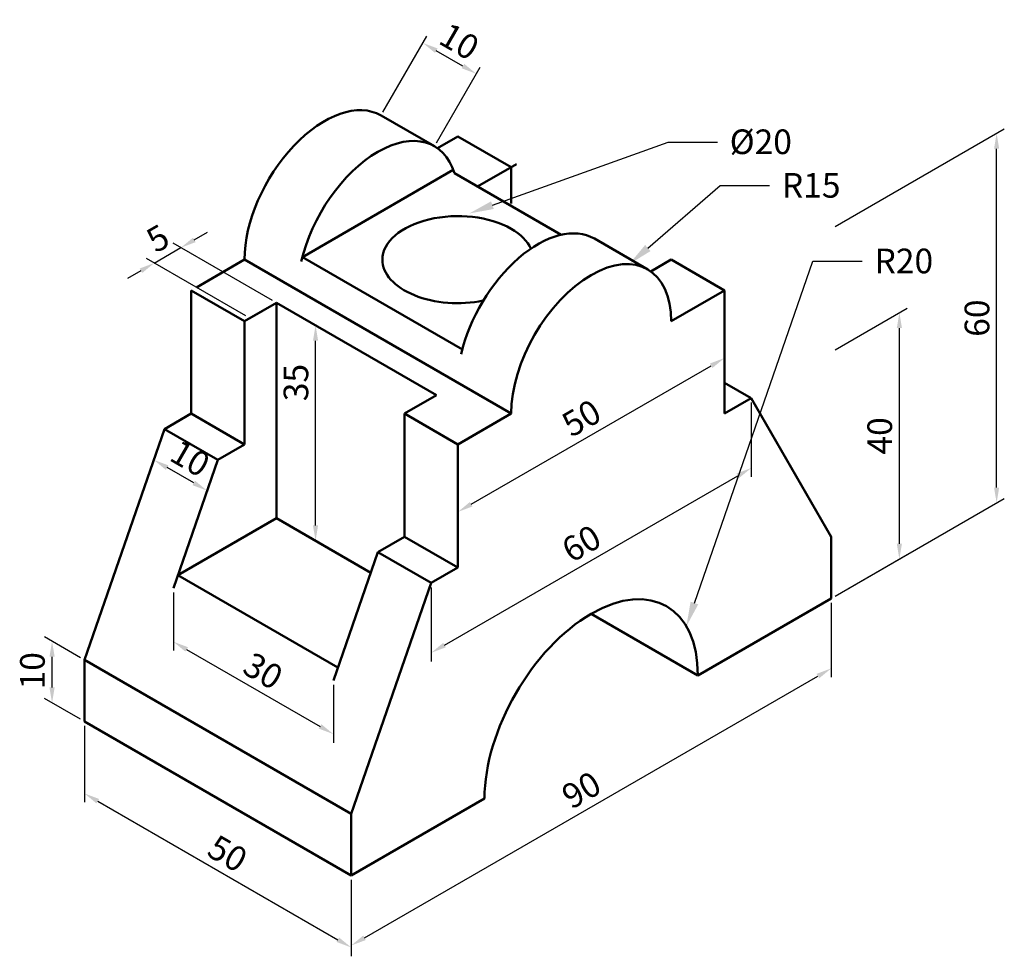
# Model space of a CAD drawing. Units: millimetres. Extents: x 1718 to 1878, y 1929 to 2081.
import ezdxf
from ezdxf import colors
from ezdxf.entities.mleader import LeaderData, LeaderLine
from ezdxf.math import Vec2, Vec3

# ---------------------------------------------------------------- set-up
doc = ezdxf.new("R2010")
doc.units = ezdxf.units.MM
for name, color, linetype, lineweight in [('M-DIMS', 2, 'Continuous', 25), ('M-OUTL', 7, 'Continuous', 50), ('M-TEXT', 3, 'Continuous', 25)]:
    doc.layers.add(name, color=color, linetype=linetype, lineweight=lineweight)
doc.styles.get("Standard").update_dxf_attribs({"font": 'arial.ttf'})
doc.dimstyles.new('ISO-25', dxfattribs={"dimtxt": 4, "dimasz": 2.5, "dimexe": 1.25, "dimexo": 0.625, "dimtad": 1, "dimtxsty": 'Standard', "dimcen": 2.5, "dimadec": 0, "dimazin": 0, "dimtfac": 1, "dimtmove": 0, "dimatfit": 3, "dimfxl": 1, "dimarcsym": 0})

# ---------------------------------------------------------------- blocks, each defined once
blk = doc.blocks.new('*D1')
at = {"layer": 'Defpoints', "color": 0, "transparency": 16777216}
for p in [(1729.01, 1966.68), (1772.31, 1941.68), (1772.31, 1930)]:
    blk.add_point(p, dxfattribs=at)
at = {"layer": 'M-DIMS', "color": 0, "lineweight": -2, "transparency": 16777216}
for p, q in [((1729.01, 1965.96), (1729.01, 1953.56)), ((1731.17, 1953.75), (1770.14, 1931.25)), ((1772.31, 1940.96), (1772.31, 1928.56))]:
    blk.add_line(p, q, dxfattribs=at)
at = {"layer": 'M-DIMS', "color": 0, "transparency": 16777216}
for points in [[(1731.38, 1954.11), (1730.96, 1953.39), (1729.01, 1955)], [(1770.35, 1931.61), (1769.93, 1930.89), (1772.31, 1930)]]:
    blk.add_solid(points, dxfattribs=at)
at = {"layer": 'M-DIMS', "color": 0, "transparency": 16777216, "insert": (1751.99, 1944.81), "char_height": 4, "attachment_point": 5, "rotation": 330}
blk.add_mtext('50', dxfattribs=at)
blk = doc.blocks.new('*D2')
at = {"layer": 'Defpoints', "color": 0, "transparency": 16777216}
for p in [(1850.25, 1986.68), (1850.25, 1975.31), (1772.31, 1941.68)]:
    blk.add_point(p, dxfattribs=at)
at = {"layer": 'M-DIMS', "color": 0, "lineweight": -2, "transparency": 16777216}
for p, q in [((1850.25, 1985.96), (1850.25, 1973.87)), ((1774.47, 1931.56), (1848.08, 1974.06)), ((1772.31, 1940.96), (1772.31, 1928.87))]:
    blk.add_line(p, q, dxfattribs=at)
at = {"layer": 'M-DIMS', "color": 0, "transparency": 16777216}
for points in [[(1847.88, 1974.42), (1848.29, 1973.7), (1850.25, 1975.31)], [(1774.26, 1931.92), (1774.68, 1931.2), (1772.31, 1930.31)]]:
    blk.add_solid(points, dxfattribs=at)
at = {"layer": 'M-DIMS', "color": 0, "transparency": 16777216, "insert": (1809.94, 1955.12), "char_height": 4, "attachment_point": 5, "rotation": 30}
blk.add_mtext('90', dxfattribs=at)
blk = doc.blocks.new('*D3')
at = {"layer": 'Defpoints', "color": 0, "transparency": 16777216}
for p in [(1723.75, 1979.71), (1729.01, 1976.68), (1729.01, 1966.68)]:
    blk.add_point(p, dxfattribs=at)
at = {"layer": 'M-DIMS', "color": 0, "lineweight": -2, "transparency": 16777216}
for p, q in [((1728.38, 1977.04), (1722.5, 1980.43)), ((1723.75, 1972.21), (1723.75, 1977.21)), ((1728.38, 1967.04), (1722.5, 1970.43))]:
    blk.add_line(p, q, dxfattribs=at)
at = {"layer": 'M-DIMS', "color": 0, "transparency": 16777216}
for points in [[(1723.33, 1977.21), (1724.17, 1977.21), (1723.75, 1979.71)], [(1723.33, 1972.21), (1724.17, 1972.21), (1723.75, 1969.71)]]:
    blk.add_solid(points, dxfattribs=at)
at = {"layer": 'M-DIMS', "color": 0, "transparency": 16777216, "insert": (1721.08, 1974.92), "char_height": 4, "attachment_point": 5, "rotation": 90}
blk.add_mtext('10', dxfattribs=at)
blk = doc.blocks.new('*D4')
at = {"layer": 'Defpoints', "color": 0, "transparency": 16777216}
for p in [(1877.1, 2062.18), (1850.25, 2046.68), (1850.25, 1986.68)]:
    blk.add_point(p, dxfattribs=at)
at = {"layer": 'M-DIMS', "color": 0, "lineweight": -2, "transparency": 16777216}
for p, q in [((1850.87, 2047.04), (1878.35, 2062.9)), ((1877.1, 2004.68), (1877.1, 2059.68)), ((1850.87, 1987.04), (1878.35, 2002.9))]:
    blk.add_line(p, q, dxfattribs=at)
at = {"layer": 'M-DIMS', "color": 0, "transparency": 16777216}
for points in [[(1876.68, 2059.68), (1877.51, 2059.68), (1877.1, 2062.18)], [(1876.68, 2004.68), (1877.51, 2004.68), (1877.1, 2002.18)]]:
    blk.add_solid(points, dxfattribs=at)
at = {"layer": 'M-DIMS', "color": 0, "transparency": 16777216, "insert": (1874.43, 2032.18), "char_height": 4, "attachment_point": 5, "rotation": 90}
blk.add_mtext('60', dxfattribs=at)
blk = doc.blocks.new('*D5')
at = {"layer": 'Defpoints', "color": 0, "transparency": 16777216}
for p in [(1861.31, 2033.06), (1850.25, 2026.68), (1850.25, 1986.68)]:
    blk.add_point(p, dxfattribs=at)
at = {"layer": 'M-DIMS', "color": 0, "lineweight": -2, "transparency": 16777216}
for p, q in [((1850.87, 2027.04), (1862.56, 2033.79)), ((1861.31, 1995.56), (1861.31, 2030.56)), ((1850.87, 1987.04), (1862.56, 1993.79))]:
    blk.add_line(p, q, dxfattribs=at)
at = {"layer": 'M-DIMS', "color": 0, "transparency": 16777216}
for points in [[(1860.89, 2030.56), (1861.73, 2030.56), (1861.31, 2033.06)], [(1860.89, 1995.56), (1861.73, 1995.56), (1861.31, 1993.06)]]:
    blk.add_solid(points, dxfattribs=at)
at = {"layer": 'M-DIMS', "color": 0, "transparency": 16777216, "insert": (1858.64, 2013.06), "char_height": 4, "attachment_point": 5, "rotation": 90}
blk.add_mtext('40', dxfattribs=at)
blk = doc.blocks.new('*D6')
at = {"layer": 'Defpoints', "color": 0, "transparency": 16777216}
for p in [(1837.26, 2019.18), (1837.26, 2007.84), (1785.3, 1989.18)]:
    blk.add_point(p, dxfattribs=at)
at = {"layer": 'M-DIMS', "color": 0, "lineweight": -2, "transparency": 16777216}
for p, q in [((1837.26, 2018.46), (1837.26, 2006.4)), ((1787.46, 1979.09), (1835.09, 2006.59)), ((1785.3, 1988.46), (1785.3, 1976.4))]:
    blk.add_line(p, q, dxfattribs=at)
at = {"layer": 'M-DIMS', "color": 0, "transparency": 16777216}
for points in [[(1834.89, 2006.95), (1835.3, 2006.23), (1837.26, 2007.84)], [(1787.25, 1979.45), (1787.67, 1978.73), (1785.3, 1977.84)]]:
    blk.add_solid(points, dxfattribs=at)
at = {"layer": 'M-DIMS', "color": 0, "transparency": 16777216, "insert": (1809.94, 1995.15), "char_height": 4, "attachment_point": 5, "rotation": 30}
blk.add_mtext('60', dxfattribs=at)
blk = doc.blocks.new('*D7')
at = {"layer": 'Defpoints', "color": 0, "transparency": 16777216}
for p in [(1832.93, 2036.68), (1832.93, 2025.71), (1789.63, 2011.68)]:
    blk.add_point(p, dxfattribs=at)
at = {"layer": 'M-DIMS', "color": 0, "lineweight": -2, "transparency": 16777216}
for p, q in [((1832.93, 2035.96), (1832.93, 2024.27)), ((1791.79, 2001.96), (1830.76, 2024.46)), ((1789.63, 2010.96), (1789.63, 1999.27))]:
    blk.add_line(p, q, dxfattribs=at)
at = {"layer": 'M-DIMS', "color": 0, "transparency": 16777216}
for points in [[(1830.56, 2024.82), (1830.97, 2024.1), (1832.93, 2025.71)], [(1791.58, 2002.32), (1792, 2001.6), (1789.63, 2000.71)]]:
    blk.add_solid(points, dxfattribs=at)
at = {"layer": 'M-DIMS', "color": 0, "transparency": 16777216, "insert": (1809.94, 2015.52), "char_height": 4, "attachment_point": 5, "rotation": 30}
blk.add_mtext('50', dxfattribs=at)
blk = doc.blocks.new('*D8')
at = {"layer": 'Defpoints', "color": 0, "transparency": 16777216}
for p in [(1744.67, 2043.63), (1760.18, 2034.68), (1755.85, 2032.18)]:
    blk.add_point(p, dxfattribs=at)
at = {"layer": 'M-DIMS', "color": 0, "lineweight": -2, "transparency": 16777216}
for p, q in [((1746.84, 2044.88), (1749, 2046.13)), ((1740.34, 2041.13), (1744.67, 2043.63)), ((1759.56, 2035.04), (1743.42, 2044.35)), ((1755.23, 2032.54), (1739.09, 2041.85)), ((1738.18, 2039.88), (1736.01, 2038.63))]:
    blk.add_line(p, q, dxfattribs=at)
at = {"layer": 'M-DIMS', "color": 0, "transparency": 16777216}
for points in [[(1746.63, 2045.24), (1747.05, 2044.52), (1744.67, 2043.63)], [(1737.97, 2040.24), (1738.39, 2039.52), (1740.34, 2041.13)]]:
    blk.add_solid(points, dxfattribs=at)
at = {"layer": 'M-DIMS', "color": 0, "transparency": 16777216, "insert": (1741.18, 2044.69), "char_height": 4, "attachment_point": 5, "rotation": 30}
blk.add_mtext('5', dxfattribs=at)
blk = doc.blocks.new('*D9')
at = {"layer": 'Defpoints', "color": 0, "transparency": 16777216}
for p in [(1743.44, 1988.35), (1769.42, 1973.35), (1769.42, 1964.64)]:
    blk.add_point(p, dxfattribs=at)
at = {"layer": 'M-DIMS', "color": 0, "lineweight": -2, "transparency": 16777216}
for p, q in [((1743.44, 1987.62), (1743.44, 1978.2)), ((1745.6, 1978.39), (1767.26, 1965.89)), ((1769.42, 1972.62), (1769.42, 1963.2))]:
    blk.add_line(p, q, dxfattribs=at)
at = {"layer": 'M-DIMS', "color": 0, "transparency": 16777216}
for points in [[(1745.81, 1978.75), (1745.4, 1978.03), (1743.44, 1979.64)], [(1767.46, 1966.25), (1767.05, 1965.53), (1769.42, 1964.64)]]:
    blk.add_solid(points, dxfattribs=at)
at = {"layer": 'M-DIMS', "color": 0, "transparency": 16777216, "insert": (1757.76, 1974.45), "char_height": 4, "attachment_point": 5, "rotation": 330}
blk.add_mtext('30', dxfattribs=at)
blk = doc.blocks.new('*D10')
at = {"layer": 'Defpoints', "color": 0, "transparency": 16777216}
for p in [(1783.96, 2076.86), (1777.16, 2065.09), (1785.82, 2060.09)]:
    blk.add_point(p, dxfattribs=at)
at = {"layer": 'M-DIMS', "color": 0, "lineweight": -2, "transparency": 16777216}
for p, q in [((1777.47, 2065.63), (1784.58, 2077.94)), ((1790.45, 2073.11), (1786.12, 2075.61)), ((1786.14, 2060.63), (1793.24, 2072.94))]:
    blk.add_line(p, q, dxfattribs=at)
at = {"layer": 'M-DIMS', "color": 0, "transparency": 16777216}
for points in [[(1786.33, 2075.97), (1785.92, 2075.25), (1783.96, 2076.86)], [(1790.66, 2073.47), (1790.25, 2072.75), (1792.62, 2071.86)]]:
    blk.add_solid(points, dxfattribs=at)
at = {"layer": 'M-DIMS', "color": 0, "transparency": 16777216, "insert": (1789.62, 2076.67), "char_height": 4, "attachment_point": 5, "rotation": 330}
blk.add_mtext('10', dxfattribs=at)
blk = doc.blocks.new('*D11')
at = {"layer": 'Defpoints', "color": 0, "transparency": 16777216}
for p in [(1760.18, 2034.68), (1766.53, 2031.02), (1760.18, 1999.68)]:
    blk.add_point(p, dxfattribs=at)
at = {"layer": 'M-DIMS', "color": 0, "lineweight": -2, "transparency": 16777216}
for p, q in [((1760.81, 2034.32), (1767.78, 2030.3)), ((1766.53, 1998.52), (1766.53, 2028.52)), ((1760.81, 1999.32), (1767.78, 1995.3))]:
    blk.add_line(p, q, dxfattribs=at)
at = {"layer": 'M-DIMS', "color": 0, "transparency": 16777216}
for points in [[(1766.11, 2028.52), (1766.94, 2028.52), (1766.53, 2031.02)], [(1766.11, 1998.52), (1766.94, 1998.52), (1766.53, 1996.02)]]:
    blk.add_solid(points, dxfattribs=at)
at = {"layer": 'M-DIMS', "color": 0, "transparency": 16777216, "insert": (1763.86, 2021.72), "char_height": 4, "attachment_point": 5, "rotation": 90}
blk.add_mtext('35', dxfattribs=at)
blk = doc.blocks.new('*D12')
at = {"layer": 'Defpoints', "color": 0, "transparency": 16777216}
for p in [(1742, 2014.18), (1740.26, 2009.17), (1750.66, 2009.18)]:
    blk.add_point(p, dxfattribs=at)
at = {"layer": 'M-DIMS', "color": 0, "lineweight": -2, "transparency": 16777216}
for p, q in [((1741.79, 2013.58), (1739.84, 2007.96)), ((1746.75, 2005.42), (1742.42, 2007.92)), ((1750.45, 2008.58), (1748.5, 2002.96))]:
    blk.add_line(p, q, dxfattribs=at)
at = {"layer": 'M-DIMS', "color": 0, "transparency": 16777216}
for points in [[(1742.63, 2008.28), (1742.22, 2007.55), (1740.26, 2009.17)], [(1746.96, 2005.78), (1746.55, 2005.05), (1748.92, 2004.17)]]:
    blk.add_solid(points, dxfattribs=at)
at = {"layer": 'M-DIMS', "color": 0, "transparency": 16777216, "insert": (1745.92, 2008.98), "char_height": 4, "attachment_point": 5, "rotation": 330}
blk.add_mtext('10', dxfattribs=at)

msp = doc.modelspace()

# ---------------------------------------------------------------- linework, layer by layer
at = {"layer": 'M-OUTL'}
for p, q in [((1777.162, 2065.089), (1785.823, 2060.089)), ((1789.628, 2061.679), (1786.32, 2059.769)), ((1798.288, 2056.679), (1789.628, 2061.679)), ((1764.39, 2042.108), (1788.885, 2056.25)), ((1789.068, 2055.71), (1806.389, 2045.71)), ((1799.154, 2057.179), (1792.839, 2053.533)), ((1798.288, 2050.821), (1798.288, 2056.679)), ((1811.803, 2045.089), (1820.464, 2040.089)), ((1747.192, 2037.179), (1754.986, 2041.679)), ((1747.192, 2037.179), (1754.986, 2041.679)), ((1754.986, 2041.679), (1798.288, 2016.679)), ((1764.39, 2042.108), (1790.371, 2027.108)), ((1824.268, 2041.679), (1820.96, 2039.769)), ((1832.929, 2036.679), (1824.268, 2041.679)), ((1754.987, 2031.679), (1746.326, 2036.679)), ((1746.326, 2036.679), (1746.326, 2016.679)), ((1832.929, 2036.679), (1824.268, 2031.679)), ((1832.929, 2036.679), (1832.929, 2016.679)), ((1760.183, 2034.679), (1754.987, 2031.679)), ((1760.183, 2034.679), (1755.852, 2032.179)), ((1786.163, 2019.679), (1760.183, 2034.679)), ((1760.183, 2034.679), (1760.183, 1999.679)), ((1754.987, 2031.679), (1754.987, 2011.679)), ((1837.259, 2019.179), (1832.929, 2021.679)), ((1780.967, 2016.679), (1786.163, 2019.679)), ((1832.929, 2016.679), (1837.259, 2019.179)), ((1837.259, 2019.179), (1850.249, 1996.679)), ((1741.996, 2014.179), (1746.326, 2016.679)), ((1746.326, 2016.679), (1754.986, 2011.679)), ((1789.627, 2011.679), (1780.967, 2016.679)), ((1780.967, 2016.679), (1780.967, 1996.679)), ((1798.288, 2016.679), (1789.627, 2011.679)), ((1741.996, 2014.179), (1729.006, 1976.679)), ((1750.656, 2009.179), (1741.996, 2014.179)), ((1754.986, 2011.679), (1750.656, 2009.179)), ((1789.627, 2011.679), (1789.627, 1991.679)), ((1750.656, 2009.179), (1743.439, 1988.346)), ((1744.161, 1990.429), (1760.183, 1999.679)), ((1775.482, 1990.846), (1760.183, 1999.679)), ((1776.637, 1994.179), (1780.967, 1996.679)), ((1780.967, 1996.679), (1789.627, 1991.679)), ((1850.249, 1986.679), (1850.249, 1996.679)), ((1776.637, 1994.179), (1769.42, 1973.346)), ((1785.297, 1989.179), (1776.637, 1994.179)), ((1770.142, 1975.429), (1744.161, 1990.429)), ((1789.627, 1991.679), (1785.297, 1989.179)), ((1785.297, 1989.179), (1772.307, 1951.679)), ((1828.599, 1974.179), (1850.249, 1986.679)), ((1828.599, 1974.179), (1811.278, 1984.179)), ((1772.307, 1951.679), (1729.006, 1976.679)), ((1729.006, 1976.679), (1729.006, 1966.679)), ((1729.006, 1966.679), (1772.307, 1941.679)), ((1772.307, 1941.679), (1793.958, 1954.179)), ((1772.307, 1941.679), (1772.307, 1951.679))]:
    msp.add_line(p, q, dxfattribs=at)
for centre, major_axis, start_param, end_param in [((1767.977, 2049.179), (-9.186, -15.91), 3.1415927, 5.4977871), ((1776.637, 2044.179), (-9.186, -15.91), 2.65071, 5.2032717), ((1789.628, 2041.679), (12.247, 0), 0.7853982, 3.1415927), ((1802.618, 2029.179), (-9.186, -15.91), 3.1415927, 5.2032717), ((1789.628, 2041.679), (12.247, 0), 0.255112, 0.7853982), ((1811.278, 2024.179), (-9.186, -15.91), 2.3561945, 5.4977871), ((1789.628, 2041.679), (12.247, 0), 3.1415927, 5.0557077), ((1811.278, 1964.179), (-12.247, -21.213), 2.3561945, 5.4977871)]:
    msp.add_ellipse(centre, major_axis=major_axis, ratio=0.5773503, start_param=start_param, end_param=end_param, dxfattribs=at)

# ---------------------------------------------------------------- dimensions: what is measured, and where the dimension line sits
at = {"layer": 'M-DIMS'}
for p1, p2, distance, picture, middle in [((1785.823, 2060.089), (1777.162, 2065.089), -13.593, '*D10', (1789.623, 2076.671)), ((1850.249, 1986.679), (1850.249, 2046.679), -26.847, '*D4', (1874.429, 2032.179)), ((1755.852, 2032.179), (1760.183, 2034.679), 15.508, '*D8', (1741.18, 2044.686)), ((1789.627, 2011.679), (1832.929, 2036.679), -9.497, '*D7', (1809.944, 2015.523)), ((1850.249, 1986.679), (1850.249, 2026.679), -11.059, '*D5', (1858.641, 2013.064)), ((1785.297, 1989.179), (1837.259, 2019.179), -9.819, '*D6', (1809.944, 1995.151)), ((1750.656, 2009.179), (1741.996, 2014.179), 5.21, '*D12', (1745.923, 2008.975)), ((1743.439, 1988.346), (1769.42, 1973.346), -7.539, '*D9', (1757.764, 1974.452)), ((1772.307, 1941.679), (1850.249, 1986.679), -9.843, '*D2', (1809.944, 1955.124)), ((1729.006, 1966.679), (1772.307, 1941.679), -10.115, '*D1', (1751.99, 1944.809))]:
    dim = msp.add_aligned_dim(p1=p1, p2=p2, distance=distance, dimstyle='ISO-25', override={"dimclrd": 0, "dimclre": 0, "dimclrt": 0}, dxfattribs=at)
    dim.commit()
    dim.dimension.update_dxf_attribs({"geometry": picture, "text_midpoint": middle})
for base, p1, p2, picture, middle in [((1766.526, 2031.017), (1760.183, 1999.679), (1760.183, 2034.679), '*D11', (1766.526, 2021.724)), ((1723.751, 1979.713), (1729.006, 1966.679), (1729.006, 1976.679), '*D3', (1723.751, 1974.919))]:
    dim = msp.add_linear_dim(base=base, p1=p1, p2=p2, angle=90, dimstyle='ISO-25', override={"dimclrd": 0, "dimclre": 0, "dimclrt": 0}, dxfattribs=at)
    dim.commit()
    dim.dimension.update_dxf_attribs({"geometry": picture, "text_midpoint": middle, "dimtype": 161})

# ---------------------------------------------------------------- leaders
at = {"layer": 'M-TEXT'}
ml = msp.add_multileader_mtext('Standard', dxfattribs=at)
ml.set_content('%%C20', color=256)
ml.set_leader_properties()
ml.build(insert=Vec2(0, 0))
ctx = ml.context
ctx.base_point, ctx.plane_origin = Vec3(1831.759, 2060.739), Vec3(1791.481, 2042.103)
notes = []
notes.append((ctx, [(0, (1, 1, 0), (1823.759, 2060.739), (1, 0), 8, [(0, [(1791.481, 2049.175)], 0, [])])]))
ctx.mtext.insert, ctx.mtext.flow_direction = Vec3(1833.759, 2062.82), 5
ml = msp.add_multileader_mtext('Standard', dxfattribs=at)
ml.set_content('R15', color=256)
ml.set_leader_properties()
ml.build(insert=Vec2(0, 0))
ctx = ml.context
ctx.base_point, ctx.plane_origin = Vec3(1840.231, 2053.712), Vec3(1817.439, 2040.942)
notes.append((ctx, [(0, (1, 1, 0), (1832.231, 2053.712), (1, 0), 8, [(0, [(1817.439, 2040.942)], 0, [])])]))
ctx.mtext.insert, ctx.mtext.flow_direction = Vec3(1842.231, 2055.746), 5
ml = msp.add_multileader_mtext('Standard', dxfattribs=at)
ml.set_content('R20', color=256)
ml.set_leader_properties()
ml.build(insert=Vec2(0, 0))
ctx = ml.context
ctx.base_point, ctx.plane_origin = Vec3(1855.272, 2041.433), Vec3(1826.728, 1982.14)
notes.append((ctx, [(0, (1, 1, 0), (1847.272, 2041.433), (1, 0), 8, [(0, [(1826.728, 1982.14)], 0, [])])]))
ctx.mtext.insert, ctx.mtext.flow_direction = Vec3(1857.272, 2043.467), 5
for ctx, leaders in notes:
    for number, flags, end, landing, length, lines in leaders:
        leader = LeaderData()
        leader.index, (leader.has_last_leader_line, leader.has_dogleg_vector, leader.attachment_direction) = number, flags
        leader.last_leader_point, leader.dogleg_vector, leader.dogleg_length = Vec3(end), Vec3(landing), length
        for number, points, colour, breaks in lines:
            line = LeaderLine()
            line.index, line.vertices, line.color, line.breaks = number, Vec3.list(points), colors.encode_raw_color(colour), breaks
            leader.lines.append(line)
        ctx.leaders.append(leader)

doc.saveas('drawing.dxf')
